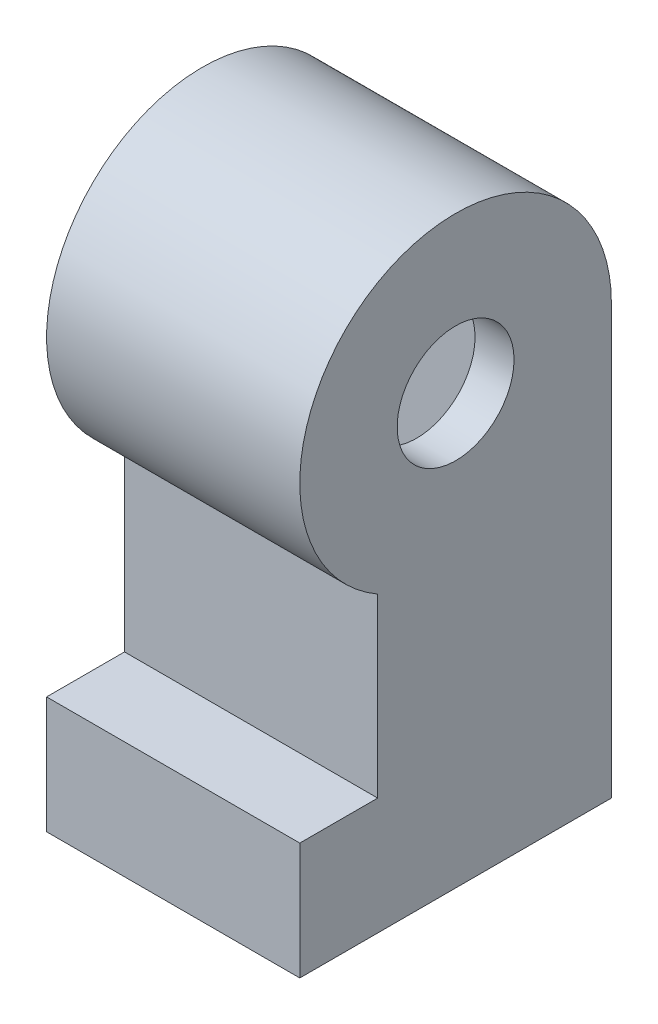
from build123d import *

# Parameters (mm, degrees)
LEG_BODY_DEPTH        = 6.5
LEG_SHELL_1MM_T       = -1
HIP_PIN_HOLE_REACH    = 15.388
HIP_PIN_HOLE_SKETCH_R = 1.5


with BuildPart() as part:
    # Leg Profile Sketch → Leg Body (new body)
    with BuildSketch(Plane(origin=(0, 0, 0), x_dir=(0, 0, -1), z_dir=(1, 0, 0))):
        with BuildLine():
            Line((4, 0), (4, -11))
            Line((4, -11), (-4, -11))
            Line((-4, -11), (-4, -8))
            Line((-4, -8), (-2, -8))
            Line((-2, -8), (-2, -3.464101615))
            ThreePointArc((-2, -3.464101615), (-2, 3.464101615), (4, 0))
        make_face()
    extrude(amount=LEG_BODY_DEPTH)

    # Leg Shell 1mm
    leg_shell_1mm_openings = [part.faces().sort_by_distance(p)[0] for p in [
        (3.25, -11, 0),
    ]]
    offset(amount=LEG_SHELL_1MM_T, openings=leg_shell_1mm_openings, kind=Kind.INTERSECTION)

    # Hip Pin Hole Sketch → Hip Pin Hole (cut, up to next)
    with BuildSketch(Plane(origin=(6.5, 0, 0), x_dir=(0, 0, -1), z_dir=(1, 0, 0)), mode=Mode.PRIVATE) as hip_pin_hole_sk1:
        Circle(HIP_PIN_HOLE_SKETCH_R)
    hip_pin_hole_tool1 = extrude(hip_pin_hole_sk1.sketch, amount=-HIP_PIN_HOLE_REACH, mode=Mode.PRIVATE) & part.part
    add(hip_pin_hole_tool1.solids().sort_by_distance((6.5, 0, 0))[0], mode=Mode.SUBTRACT)


solid = part.part
